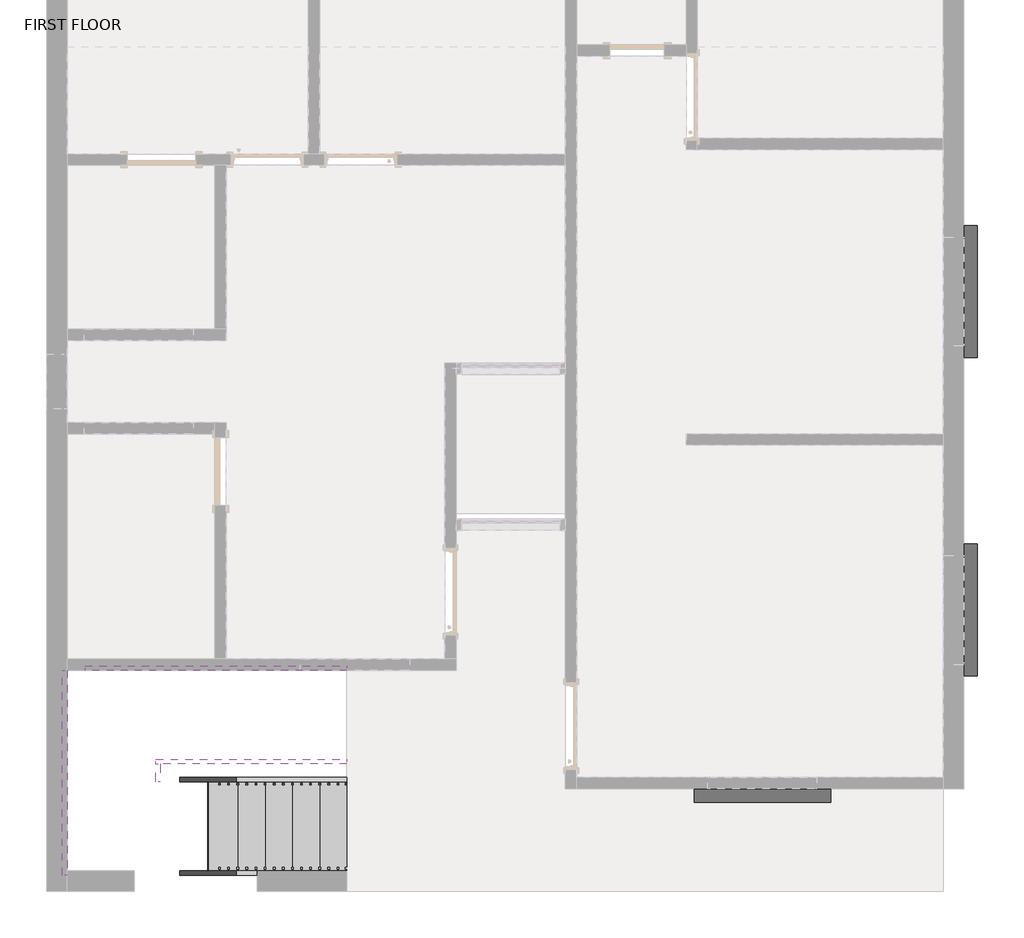
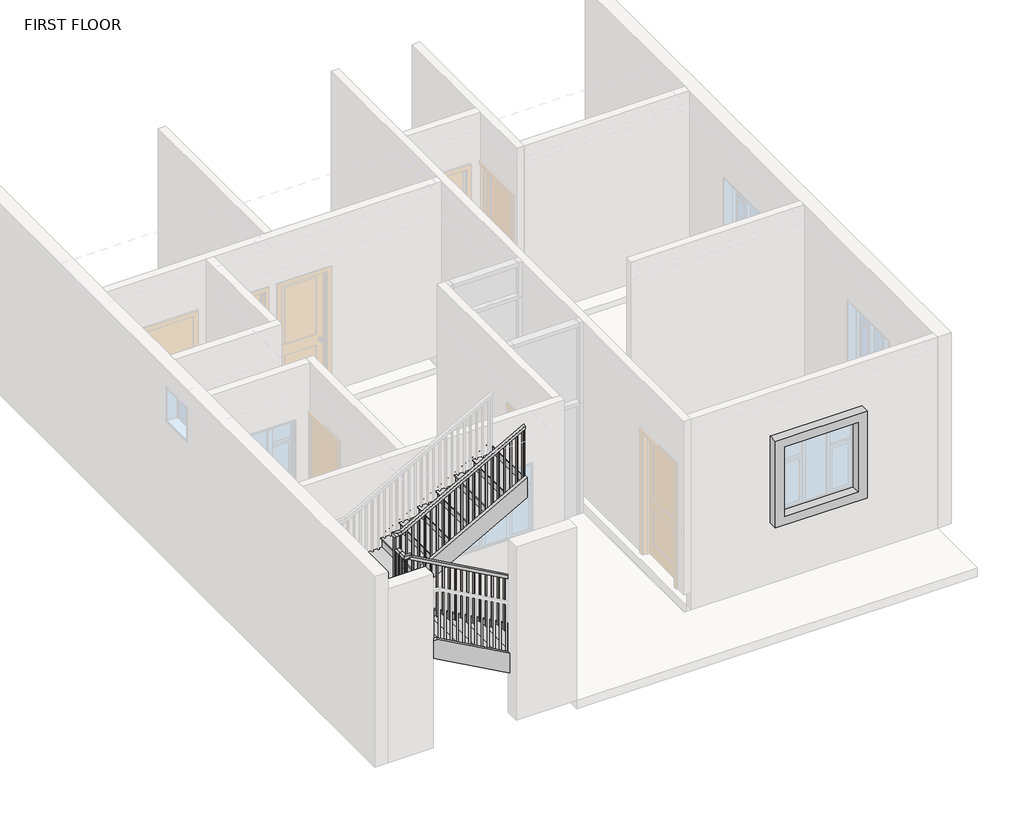
# One storey, part 3 of 3: 6 members, 3 proxies, 1 railing, 1 stair flight.
"""IFC4 building model written with IfcOpenShell, lengths in millimetres."""

from ifc_helpers import new_model, si_unit, frame, origin, place, context, project, spatial, polyline, outline, extrude, faceted_brep, transform, mapped, element, save
from components import generic_models_3_generic_models_3_0ad4c425, generic_models_6_generic_models_6_ceaf88ca, stair_flight_128b20ea

model = new_model("IFC4")

# Units and contexts
model_context = context("Model", 3, world=origin())
ifc_project = project(units=[si_unit("LENGTHUNIT", "METRE", prefix="MILLI")], contexts=[model_context])

# Site, building, storey
site = spatial("IfcSite", under=ifc_project)
building = spatial("IfcBuilding", under=site)
storey = spatial("IfcBuildingStorey", under=building, Name="FIRST FLOOR", Elevation=3352.8)

# Proxies
placement = place(None, origin())
generic_models_3_generic_models_3_shape = generic_models_3_generic_models_3_0ad4c425(model_context)
element("IfcBuildingElementProxy", 1, Name="Generic Models 3 : Generic Models 3", ObjectType="Generic Models 3 : Generic Models 3", at=placement, inside=storey, context=model_context, shape_type="MappedRepresentation", body=[
    mapped(generic_models_3_generic_models_3_shape, transform((0.0, 0.0, 0.0), x_axis=(1.0, 0.0, 0.0), y_axis=(0.0, 1.0, 0.0), z_axis=(0.0, 0.0, 1.0))),
])
generic_models_6_generic_models_6_shape = generic_models_6_generic_models_6_ceaf88ca(model_context)
element("IfcBuildingElementProxy", 2, Name="Generic Models 6 : Generic Models 6", ObjectType="Generic Models 6 : Generic Models 6", at=placement, inside=storey, context=model_context, shape_type="MappedRepresentation", body=[
    mapped(generic_models_6_generic_models_6_shape, transform((0.0, 0.0, 0.0), x_axis=(1.0, 0.0, 0.0), y_axis=(0.0, 1.0, 0.0), z_axis=(0.0, 0.0, 1.0))),
])
element("IfcBuildingElementProxy", 3, Name="Generic Models 7 : Generic Models 6", ObjectType="Generic Models 7 : Generic Models 6", at=placement, inside=storey, context=model_context, shape_type="MappedRepresentation", body=[
    mapped(generic_models_6_generic_models_6_shape, transform((0.0, 3556.0, 0.0), x_axis=(1.0, 0.0, 0.0), y_axis=(0.0, 1.0, 0.0), z_axis=(0.0, 0.0, 1.0))),
])

# Members
element("IfcMember", 4, ObjectType="Stringer - 2\" Width", at=placement, inside=storey, context=model_context, shape_type="SweptSolid", body=[
    extrude(outline(polyline([(3657.6, -11636.5023867), (3865.1983948, -11636.5023867), (5088.4666667, -13838.3852761), (5088.4666667, -14466.0068895), (3657.6, -11890.4468895), (3657.6, -11636.5023867)])), frame((0.0, -2807.5499863, 0.0), z_axis=(0.0, 1.0, 0.0), x_axis=(0.0, 0.0, 1.0)), (0.0, 0.0, 1.0), 50.8),
])
element("IfcMember", 5, ObjectType="Stringer - 2\" Width", at=placement, inside=storey, context=model_context, shape_type="SweptSolid", body=[
    extrude(outline(polyline([(-14760.7023867, -2807.5499863), (-14811.5023867, -2807.5499863), (-14811.5023867, -521.5499863), (-14760.7023867, -521.5499863), (-14760.7023867, -2807.5499863)])), frame((0.0, 0.0, 4783.6666667), z_axis=(0.0, 0.0, 1.0), x_axis=(1.0, 0.0, 0.0)), (0.0, 0.0, 1.0), 304.8),
])
element("IfcMember", 6, ObjectType="Stringer - 2\" Width", at=placement, inside=storey, context=model_context, shape_type="SweptSolid", body=[
    extrude(outline(polyline([(4783.6666667, -13927.6378839), (6056.5197207, -11636.5023867), (6405.1983948, -11636.5023867), (4783.6666667, -14555.2594973), (4783.6666667, -13927.6378839)])), frame((0.0, -521.5499863, 0.0), z_axis=(0.0, 1.0, 0.0), x_axis=(0.0, 0.0, 1.0)), (0.0, 0.0, 1.0), 50.8),
])
element("IfcMember", 7, ObjectType="Stringer - 2\" Width", at=placement, inside=storey, context=model_context, shape_type="SweptSolid", body=[
    extrude(outline(polyline([(3657.6, -11636.5023867), (3865.1983948, -11636.5023867), (5022.3095059, -13719.3023867), (4673.6308318, -13719.3023867), (3657.6, -11890.4468895), (3657.6, -11636.5023867)])), frame((0.0, -1766.1499863, 0.0), z_axis=(0.0, 1.0, 0.0), x_axis=(0.0, 0.0, 1.0)), (0.0, 0.0, 1.0), 50.8),
])
element("IfcMember", 8, ObjectType="Stringer - 2\" Width", at=placement, inside=storey, context=model_context, shape_type="SweptSolid", body=[
    extrude(outline(polyline([(-13719.3023867, -1766.1499863), (-13770.1023867, -1766.1499863), (-13770.1023867, -1562.9499863), (-13719.3023867, -1562.9499863), (-13719.3023867, -1766.1499863)])), frame((0.0, 0.0, 4783.6666667), z_axis=(0.0, 0.0, 1.0), x_axis=(1.0, 0.0, 0.0)), (0.0, 0.0, 1.0), 304.8),
])
element("IfcMember", 9, ObjectType="Stringer - 2\" Width", at=placement, inside=storey, context=model_context, shape_type="SweptSolid", body=[
    extrude(outline(polyline([(5219.8650614, -13770.1023867), (4871.1863873, -13770.1023867), (6056.5197207, -11636.5023867), (6405.1983948, -11636.5023867), (5219.8650614, -13770.1023867)])), frame((0.0, -1562.9499863, 0.0), z_axis=(0.0, 1.0, 0.0), x_axis=(0.0, 0.0, 1.0)), (0.0, 0.0, 1.0), 50.8),
])

# Railing
element("IfcRailing", 10, ObjectType="Handrail - Rectangular", at=placement, inside=storey, context=model_context, shape_type="SolidModel", body=[
    faceted_brep([(-11636.5023867, -1816.9499863, 4741.3333333), (-11636.5023867, -1816.9499863, 4683.220221), (-11636.5023867, -1766.1499863, 4683.220221), (-11636.5023867, -1766.1499863, 4741.3333333), (-13693.9023867, -1816.9499863, 5884.3333333), (-13744.7023867, -1816.9499863, 5854.4424432), (-13744.7023867, -1766.1499863, 5854.4424432), (-13693.9023867, -1766.1499863, 5884.3333333), (-13693.9023867, -1816.9499863, 5926.6666667), (-13744.7023867, -1816.9499863, 5875.8666667), (-13744.7023867, -1766.1499863, 5875.8666667), (-13693.9023867, -1766.1499863, 5926.6666667), (-13820.9023867, -1816.9499863, 5926.6666667), (-13820.9023867, -1816.9499863, 5875.8666667), (-13770.1023867, -1766.1499863, 5875.8666667), (-13770.1023867, -1766.1499863, 5926.6666667), (-13820.9023867, -1689.9499863, 5926.6666667), (-13820.9023867, -1689.9499863, 5875.8666667), (-13770.1023867, -1689.9499863, 5875.8666667), (-13770.1023867, -1689.9499863, 5926.6666667), (-13820.9023867, -1588.3499863, 5926.6666667), (-13820.9023867, -1537.5499863, 5875.8666667), (-13770.1023867, -1537.5499863, 5875.8666667), (-13770.1023867, -1588.3499863, 5926.6666667), (-13820.9023867, -1588.3499863, 6138.3333333), (-13820.9023867, -1537.5499863, 6087.5333333), (-13770.1023867, -1537.5499863, 6087.5333333), (-13770.1023867, -1588.3499863, 6138.3333333), (-13820.9023867, -1461.3499863, 6138.3333333), (-13820.9023867, -1461.3499863, 6087.5333333), (-13770.1023867, -1512.1499863, 6087.5333333), (-13770.1023867, -1512.1499863, 6138.3333333), (-13693.9023867, -1461.3499863, 6138.3333333), (-13680.7387844, -1461.3499863, 6087.5333333), (-13680.7387844, -1512.1499863, 6087.5333333), (-13693.9023867, -1512.1499863, 6138.3333333), (-11636.5023867, -1461.3499863, 7281.3333333), (-11636.5023867, -1512.1499863, 7281.3333333), (-11636.5023867, -1512.1499863, 7223.220221), (-11636.5023867, -1461.3499863, 7223.220221)], [[[0, 1, 2, 3]], [[1, 0, 4, 5]], [[2, 1, 5, 6]], [[3, 2, 6, 7]], [[0, 3, 7, 4]], [[5, 4, 8, 9]], [[6, 5, 9, 10]], [[7, 6, 10, 11]], [[4, 7, 11, 8]], [[9, 8, 12, 13]], [[10, 9, 13, 14]], [[11, 10, 14, 15]], [[8, 11, 15, 12]], [[13, 12, 16, 17]], [[14, 13, 17, 18]], [[15, 14, 18, 19]], [[12, 15, 19, 16]], [[17, 16, 20, 21]], [[18, 17, 21, 22]], [[19, 18, 22, 23]], [[16, 19, 23, 20]], [[21, 20, 24, 25]], [[22, 21, 25, 26]], [[23, 22, 26, 27]], [[20, 23, 27, 24]], [[25, 24, 28, 29]], [[26, 25, 29, 30]], [[27, 26, 30, 31]], [[24, 27, 31, 28]], [[29, 28, 32, 33]], [[30, 29, 33, 34]], [[31, 30, 34, 35]], [[28, 31, 35, 32]], [[36, 37, 38, 39]], [[33, 32, 36, 39]], [[34, 33, 39, 38]], [[35, 34, 38, 37]], [[32, 35, 37, 36]]]),
    extrude(outline(polyline([(7214.4007765, -11652.3773867), (7203.8174432, -11671.4273867), (6197.6, -11671.4273867), (6197.6, -11652.3773867), (7214.4007765, -11652.3773867)])), frame((0.0, -1496.2749863, 0.0), z_axis=(0.0, 1.0, 0.0), x_axis=(0.0, 0.0, 1.0)), (0.0, 0.0, 1.0), 19.05),
    extrude(outline(polyline([(7157.9563321, -11753.9773867), (7147.3729988, -11773.0273867), (6197.6, -11773.0273867), (6197.6, -11753.9773867), (7157.9563321, -11753.9773867)])), frame((0.0, -1496.2749863, 0.0), z_axis=(0.0, 1.0, 0.0), x_axis=(0.0, 0.0, 1.0)), (0.0, 0.0, 1.0), 19.05),
    extrude(outline(polyline([(7101.5118876, -11855.5773867), (7090.9285543, -11874.6273867), (6197.6, -11874.6273867), (6197.6, -11855.5773867), (7101.5118876, -11855.5773867)])), frame((0.0, -1496.2749863, 0.0), z_axis=(0.0, 1.0, 0.0), x_axis=(0.0, 0.0, 1.0)), (0.0, 0.0, 1.0), 19.05),
    extrude(outline(polyline([(7045.0674432, -11957.1773867), (7034.4841099, -11976.2273867), (6028.2666667, -11976.2273867), (6028.2666667, -11957.1773867), (7045.0674432, -11957.1773867)])), frame((0.0, -1496.2749863, 0.0), z_axis=(0.0, 1.0, 0.0), x_axis=(0.0, 0.0, 1.0)), (0.0, 0.0, 1.0), 19.05),
    extrude(outline(polyline([(6988.6229988, -12058.7773867), (6978.0396654, -12077.8273867), (6028.2666667, -12077.8273867), (6028.2666667, -12058.7773867), (6988.6229988, -12058.7773867)])), frame((0.0, -1496.2749863, 0.0), z_axis=(0.0, 1.0, 0.0), x_axis=(0.0, 0.0, 1.0)), (0.0, 0.0, 1.0), 19.05),
    extrude(outline(polyline([(6932.1785543, -12160.3773867), (6921.595221, -12179.4273867), (6028.2666667, -12179.4273867), (6028.2666667, -12160.3773867), (6932.1785543, -12160.3773867)])), frame((0.0, -1496.2749863, 0.0), z_axis=(0.0, 1.0, 0.0), x_axis=(0.0, 0.0, 1.0)), (0.0, 0.0, 1.0), 19.05),
    extrude(outline(polyline([(6875.7341099, -12261.9773867), (6865.1507765, -12281.0273867), (5858.9333333, -12281.0273867), (5858.9333333, -12261.9773867), (6875.7341099, -12261.9773867)])), frame((0.0, -1496.2749863, 0.0), z_axis=(0.0, 1.0, 0.0), x_axis=(0.0, 0.0, 1.0)), (0.0, 0.0, 1.0), 19.05),
    extrude(outline(polyline([(6819.2896654, -12363.5773867), (6808.7063321, -12382.6273867), (5858.9333333, -12382.6273867), (5858.9333333, -12363.5773867), (6819.2896654, -12363.5773867)])), frame((0.0, -1496.2749863, 0.0), z_axis=(0.0, 1.0, 0.0), x_axis=(0.0, 0.0, 1.0)), (0.0, 0.0, 1.0), 19.05),
    extrude(outline(polyline([(6762.845221, -12465.1773867), (6752.2618876, -12484.2273867), (5858.9333333, -12484.2273867), (5858.9333333, -12465.1773867), (6762.845221, -12465.1773867)])), frame((0.0, -1496.2749863, 0.0), z_axis=(0.0, 1.0, 0.0), x_axis=(0.0, 0.0, 1.0)), (0.0, 0.0, 1.0), 19.05),
    extrude(outline(polyline([(6706.4007765, -12566.7773867), (6695.8174432, -12585.8273867), (5689.6, -12585.8273867), (5689.6, -12566.7773867), (6706.4007765, -12566.7773867)])), frame((0.0, -1496.2749863, 0.0), z_axis=(0.0, 1.0, 0.0), x_axis=(0.0, 0.0, 1.0)), (0.0, 0.0, 1.0), 19.05),
    extrude(outline(polyline([(6649.9563321, -12668.3773867), (6639.3729988, -12687.4273867), (5689.6, -12687.4273867), (5689.6, -12668.3773867), (6649.9563321, -12668.3773867)])), frame((0.0, -1496.2749863, 0.0), z_axis=(0.0, 1.0, 0.0), x_axis=(0.0, 0.0, 1.0)), (0.0, 0.0, 1.0), 19.05),
    extrude(outline(polyline([(6593.5118876, -12769.9773867), (6582.9285543, -12789.0273867), (5689.6, -12789.0273867), (5689.6, -12769.9773867), (6593.5118876, -12769.9773867)])), frame((0.0, -1496.2749863, 0.0), z_axis=(0.0, 1.0, 0.0), x_axis=(0.0, 0.0, 1.0)), (0.0, 0.0, 1.0), 19.05),
    extrude(outline(polyline([(6537.0674432, -12871.5773867), (6526.4841099, -12890.6273867), (5520.2666667, -12890.6273867), (5520.2666667, -12871.5773867), (6537.0674432, -12871.5773867)])), frame((0.0, -1496.2749863, 0.0), z_axis=(0.0, 1.0, 0.0), x_axis=(0.0, 0.0, 1.0)), (0.0, 0.0, 1.0), 19.05),
    extrude(outline(polyline([(6480.6229988, -12973.1773867), (6470.0396654, -12992.2273867), (5520.2666667, -12992.2273867), (5520.2666667, -12973.1773867), (6480.6229988, -12973.1773867)])), frame((0.0, -1496.2749863, 0.0), z_axis=(0.0, 1.0, 0.0), x_axis=(0.0, 0.0, 1.0)), (0.0, 0.0, 1.0), 19.05),
    extrude(outline(polyline([(6424.1785543, -13074.7773867), (6413.595221, -13093.8273867), (5520.2666667, -13093.8273867), (5520.2666667, -13074.7773867), (6424.1785543, -13074.7773867)])), frame((0.0, -1496.2749863, 0.0), z_axis=(0.0, 1.0, 0.0), x_axis=(0.0, 0.0, 1.0)), (0.0, 0.0, 1.0), 19.05),
    extrude(outline(polyline([(6367.7341099, -13176.3773867), (6357.1507765, -13195.4273867), (5350.9333333, -13195.4273867), (5350.9333333, -13176.3773867), (6367.7341099, -13176.3773867)])), frame((0.0, -1496.2749863, 0.0), z_axis=(0.0, 1.0, 0.0), x_axis=(0.0, 0.0, 1.0)), (0.0, 0.0, 1.0), 19.05),
    extrude(outline(polyline([(6311.2896654, -13277.9773867), (6300.7063321, -13297.0273867), (5350.9333333, -13297.0273867), (5350.9333333, -13277.9773867), (6311.2896654, -13277.9773867)])), frame((0.0, -1496.2749863, 0.0), z_axis=(0.0, 1.0, 0.0), x_axis=(0.0, 0.0, 1.0)), (0.0, 0.0, 1.0), 19.05),
    extrude(outline(polyline([(6254.845221, -13379.5773867), (6244.2618876, -13398.6273867), (5350.9333333, -13398.6273867), (5350.9333333, -13379.5773867), (6254.845221, -13379.5773867)])), frame((0.0, -1496.2749863, 0.0), z_axis=(0.0, 1.0, 0.0), x_axis=(0.0, 0.0, 1.0)), (0.0, 0.0, 1.0), 19.05),
    extrude(outline(polyline([(6198.4007765, -13481.1773867), (6187.8174432, -13500.2273867), (5181.6, -13500.2273867), (5181.6, -13481.1773867), (6198.4007765, -13481.1773867)])), frame((0.0, -1496.2749863, 0.0), z_axis=(0.0, 1.0, 0.0), x_axis=(0.0, 0.0, 1.0)), (0.0, 0.0, 1.0), 19.05),
    extrude(outline(polyline([(6141.9563321, -13582.7773867), (6131.3729988, -13601.8273867), (5181.6, -13601.8273867), (5181.6, -13582.7773867), (6141.9563321, -13582.7773867)])), frame((0.0, -1496.2749863, 0.0), z_axis=(0.0, 1.0, 0.0), x_axis=(0.0, 0.0, 1.0)), (0.0, 0.0, 1.0), 19.05),
    extrude(outline(polyline([(6085.5118876, -13684.3773867), (6074.9285543, -13703.4273867), (5181.6, -13703.4273867), (5181.6, -13684.3773867), (6085.5118876, -13684.3773867)])), frame((0.0, -1496.2749863, 0.0), z_axis=(0.0, 1.0, 0.0), x_axis=(0.0, 0.0, 1.0)), (0.0, 0.0, 1.0), 19.05),
    extrude(outline(polyline([(-13785.9773867, -1597.8749863), (-13805.0273867, -1597.8749863), (-13805.0273867, -1578.8249863), (-13785.9773867, -1578.8249863), (-13785.9773867, -1597.8749863)])), frame((0.0, 0.0, 5012.2666667), z_axis=(0.0, 0.0, 1.0), x_axis=(1.0, 0.0, 0.0)), (0.0, 0.0, 1.0), 863.6),
    extrude(outline(polyline([(-13785.9773867, -1699.4749863), (-13805.0273867, -1699.4749863), (-13805.0273867, -1680.4249863), (-13785.9773867, -1680.4249863), (-13785.9773867, -1699.4749863)])), frame((0.0, 0.0, 5012.2666667), z_axis=(0.0, 0.0, 1.0), x_axis=(1.0, 0.0, 0.0)), (0.0, 0.0, 1.0), 863.6),
    extrude(outline(polyline([(-13760.5773867, -1782.0249863), (-13760.5773867, -1801.0749863), (-13779.6273867, -1801.0749863), (-13779.6273867, -1782.0249863), (-13760.5773867, -1782.0249863)])), frame((0.0, 0.0, 5012.2666667), z_axis=(0.0, 0.0, 1.0), x_axis=(1.0, 0.0, 0.0)), (0.0, 0.0, 1.0), 863.6),
    extrude(outline(polyline([(5806.8174432, -13658.9773867), (5817.4007765, -13678.0273867), (4842.9333333, -13678.0273867), (4842.9333333, -13658.9773867), (5806.8174432, -13658.9773867)])), frame((0.0, -1801.0749863, 0.0), z_axis=(0.0, 1.0, 0.0), x_axis=(0.0, 0.0, 1.0)), (0.0, 0.0, 1.0), 19.05),
    extrude(outline(polyline([(5750.3729988, -13557.3773867), (5760.9563321, -13576.4273867), (4842.9333333, -13576.4273867), (4842.9333333, -13557.3773867), (5750.3729988, -13557.3773867)])), frame((0.0, -1801.0749863, 0.0), z_axis=(0.0, 1.0, 0.0), x_axis=(0.0, 0.0, 1.0)), (0.0, 0.0, 1.0), 19.05),
    extrude(outline(polyline([(5693.9285543, -13455.7773867), (5704.5118876, -13474.8273867), (4842.9333333, -13474.8273867), (4842.9333333, -13455.7773867), (5693.9285543, -13455.7773867)])), frame((0.0, -1801.0749863, 0.0), z_axis=(0.0, 1.0, 0.0), x_axis=(0.0, 0.0, 1.0)), (0.0, 0.0, 1.0), 19.05),
    extrude(outline(polyline([(5637.4841099, -13354.1773867), (5648.0674432, -13373.2273867), (4673.6, -13373.2273867), (4673.6, -13354.1773867), (5637.4841099, -13354.1773867)])), frame((0.0, -1801.0749863, 0.0), z_axis=(0.0, 1.0, 0.0), x_axis=(0.0, 0.0, 1.0)), (0.0, 0.0, 1.0), 19.05),
    extrude(outline(polyline([(5581.0396654, -13252.5773867), (5591.6229988, -13271.6273867), (4673.6, -13271.6273867), (4673.6, -13252.5773867), (5581.0396654, -13252.5773867)])), frame((0.0, -1801.0749863, 0.0), z_axis=(0.0, 1.0, 0.0), x_axis=(0.0, 0.0, 1.0)), (0.0, 0.0, 1.0), 19.05),
    extrude(outline(polyline([(5524.595221, -13150.9773867), (5535.1785543, -13170.0273867), (4673.6, -13170.0273867), (4673.6, -13150.9773867), (5524.595221, -13150.9773867)])), frame((0.0, -1801.0749863, 0.0), z_axis=(0.0, 1.0, 0.0), x_axis=(0.0, 0.0, 1.0)), (0.0, 0.0, 1.0), 19.05),
    extrude(outline(polyline([(5468.1507765, -13049.3773867), (5478.7341099, -13068.4273867), (4504.2666667, -13068.4273867), (4504.2666667, -13049.3773867), (5468.1507765, -13049.3773867)])), frame((0.0, -1801.0749863, 0.0), z_axis=(0.0, 1.0, 0.0), x_axis=(0.0, 0.0, 1.0)), (0.0, 0.0, 1.0), 19.05),
    extrude(outline(polyline([(5411.7063321, -12947.7773867), (5422.2896654, -12966.8273867), (4504.2666667, -12966.8273867), (4504.2666667, -12947.7773867), (5411.7063321, -12947.7773867)])), frame((0.0, -1801.0749863, 0.0), z_axis=(0.0, 1.0, 0.0), x_axis=(0.0, 0.0, 1.0)), (0.0, 0.0, 1.0), 19.05),
    extrude(outline(polyline([(5355.2618876, -12846.1773867), (5365.845221, -12865.2273867), (4504.2666667, -12865.2273867), (4504.2666667, -12846.1773867), (5355.2618876, -12846.1773867)])), frame((0.0, -1801.0749863, 0.0), z_axis=(0.0, 1.0, 0.0), x_axis=(0.0, 0.0, 1.0)), (0.0, 0.0, 1.0), 19.05),
    extrude(outline(polyline([(5298.8174432, -12744.5773867), (5309.4007765, -12763.6273867), (4334.9333333, -12763.6273867), (4334.9333333, -12744.5773867), (5298.8174432, -12744.5773867)])), frame((0.0, -1801.0749863, 0.0), z_axis=(0.0, 1.0, 0.0), x_axis=(0.0, 0.0, 1.0)), (0.0, 0.0, 1.0), 19.05),
    extrude(outline(polyline([(5242.3729988, -12642.9773867), (5252.9563321, -12662.0273867), (4334.9333333, -12662.0273867), (4334.9333333, -12642.9773867), (5242.3729988, -12642.9773867)])), frame((0.0, -1801.0749863, 0.0), z_axis=(0.0, 1.0, 0.0), x_axis=(0.0, 0.0, 1.0)), (0.0, 0.0, 1.0), 19.05),
    extrude(outline(polyline([(5185.9285543, -12541.3773867), (5196.5118876, -12560.4273867), (4334.9333333, -12560.4273867), (4334.9333333, -12541.3773867), (5185.9285543, -12541.3773867)])), frame((0.0, -1801.0749863, 0.0), z_axis=(0.0, 1.0, 0.0), x_axis=(0.0, 0.0, 1.0)), (0.0, 0.0, 1.0), 19.05),
    extrude(outline(polyline([(5129.4841099, -12439.7773867), (5140.0674432, -12458.8273867), (4165.6, -12458.8273867), (4165.6, -12439.7773867), (5129.4841099, -12439.7773867)])), frame((0.0, -1801.0749863, 0.0), z_axis=(0.0, 1.0, 0.0), x_axis=(0.0, 0.0, 1.0)), (0.0, 0.0, 1.0), 19.05),
    extrude(outline(polyline([(5073.0396654, -12338.1773867), (5083.6229988, -12357.2273867), (4165.6, -12357.2273867), (4165.6, -12338.1773867), (5073.0396654, -12338.1773867)])), frame((0.0, -1801.0749863, 0.0), z_axis=(0.0, 1.0, 0.0), x_axis=(0.0, 0.0, 1.0)), (0.0, 0.0, 1.0), 19.05),
    extrude(outline(polyline([(5016.595221, -12236.5773867), (5027.1785543, -12255.6273867), (4165.6, -12255.6273867), (4165.6, -12236.5773867), (5016.595221, -12236.5773867)])), frame((0.0, -1801.0749863, 0.0), z_axis=(0.0, 1.0, 0.0), x_axis=(0.0, 0.0, 1.0)), (0.0, 0.0, 1.0), 19.05),
    extrude(outline(polyline([(4960.1507765, -12134.9773867), (4970.7341099, -12154.0273867), (3996.2666667, -12154.0273867), (3996.2666667, -12134.9773867), (4960.1507765, -12134.9773867)])), frame((0.0, -1801.0749863, 0.0), z_axis=(0.0, 1.0, 0.0), x_axis=(0.0, 0.0, 1.0)), (0.0, 0.0, 1.0), 19.05),
    extrude(outline(polyline([(4903.7063321, -12033.3773867), (4914.2896654, -12052.4273867), (3996.2666667, -12052.4273867), (3996.2666667, -12033.3773867), (4903.7063321, -12033.3773867)])), frame((0.0, -1801.0749863, 0.0), z_axis=(0.0, 1.0, 0.0), x_axis=(0.0, 0.0, 1.0)), (0.0, 0.0, 1.0), 19.05),
    extrude(outline(polyline([(4847.2618876, -11931.7773867), (4857.845221, -11950.8273867), (3996.2666667, -11950.8273867), (3996.2666667, -11931.7773867), (4847.2618876, -11931.7773867)])), frame((0.0, -1801.0749863, 0.0), z_axis=(0.0, 1.0, 0.0), x_axis=(0.0, 0.0, 1.0)), (0.0, 0.0, 1.0), 19.05),
    extrude(outline(polyline([(4790.8174432, -11830.1773867), (4801.4007765, -11849.2273867), (3826.9333333, -11849.2273867), (3826.9333333, -11830.1773867), (4790.8174432, -11830.1773867)])), frame((0.0, -1801.0749863, 0.0), z_axis=(0.0, 1.0, 0.0), x_axis=(0.0, 0.0, 1.0)), (0.0, 0.0, 1.0), 19.05),
    extrude(outline(polyline([(4734.3729988, -11728.5773867), (4744.9563321, -11747.6273867), (3826.9333333, -11747.6273867), (3826.9333333, -11728.5773867), (4734.3729988, -11728.5773867)])), frame((0.0, -1801.0749863, 0.0), z_axis=(0.0, 1.0, 0.0), x_axis=(0.0, 0.0, 1.0)), (0.0, 0.0, 1.0), 19.05),
    extrude(outline(polyline([(-13785.9773867, -1496.2749863), (-13805.0273867, -1496.2749863), (-13805.0273867, -1477.2249863), (-13785.9773867, -1477.2249863), (-13785.9773867, -1496.2749863)])), frame((0.0, 0.0, 5012.2666667), z_axis=(0.0, 0.0, 1.0), x_axis=(1.0, 0.0, 0.0)), (0.0, 0.0, 1.0), 1075.2666667),
    extrude(outline(polyline([(-13785.9773867, -1782.0249863), (-13785.9773867, -1801.0749863), (-13805.0273867, -1801.0749863), (-13805.0273867, -1782.0249863), (-13785.9773867, -1782.0249863)])), frame((0.0, 0.0, 5012.2666667), z_axis=(0.0, 0.0, 1.0), x_axis=(1.0, 0.0, 0.0)), (0.0, 0.0, 1.0), 863.6),
    extrude(outline(polyline([(7223.220221, -11636.5023867), (7212.6368876, -11655.5523867), (6197.6, -11655.5523867), (6197.6, -11636.5023867), (7223.220221, -11636.5023867)])), frame((0.0, -1496.2749863, 0.0), z_axis=(0.0, 1.0, 0.0), x_axis=(0.0, 0.0, 1.0)), (0.0, 0.0, 1.0), 19.05),
    extrude(outline(polyline([(4683.220221, -11636.5023867), (4693.8035543, -11655.5523867), (3826.9333333, -11655.5523867), (3826.9333333, -11636.5023867), (4683.220221, -11636.5023867)])), frame((0.0, -1801.0749863, 0.0), z_axis=(0.0, 1.0, 0.0), x_axis=(0.0, 0.0, 1.0)), (0.0, 0.0, 1.0), 19.05),
])

# Stair flight
stair_flight_shape = stair_flight_128b20ea(model_context)
element("IfcStairFlight", 11, ObjectType="2\" Tread 1\" Nosing 1/4\" Riser", at=placement, inside=storey, context=model_context, shape_type="MappedRepresentation", body=[
    mapped(stair_flight_shape, transform((0.0, 0.0, 0.0), x_axis=(1.0, 0.0, 0.0), y_axis=(0.0, 1.0, 0.0), z_axis=(0.0, 0.0, 1.0))),
])

save(model, "model.ifc")

# Revit data of these elements
# Type "Handrail - Rectangular"
#   Assembly Code = "C2010400"
#   built-in parameter 1008612 = 0.0416667 (stored number, unit not read)
#   built-in parameter 1008611 = 0.0416667 (stored number, unit not read)
#   built-in parameter 1008609 = 0.333333 (stored number, unit not read)
#   built-in parameter 1008604 = 0.166667 (stored number, unit not read)
#   built-in parameter 1008603 = 0.166667 (stored number, unit not read)
#   Railing Height = 3' - 0"
#   built-in parameter 1008630 = 2
#   built-in parameter 1008610 = 2
#   built-in parameter 1008618 = Baluster - Square : 3/4"
# Element 1 (IfcBuildingElementProxy, "Generic Models 3 : Generic Models 3")
#   Phase Created = New Construction
#   Materials on its faces: "accent wall"
# Element 2 (IfcBuildingElementProxy, "Generic Models 6 : Generic Models 6")
#   Phase Created = New Construction
#   Materials on its faces: "accent wall"
# Element 3 (IfcBuildingElementProxy, "Generic Models 7 : Generic Models 6")
#   Phase Created = New Construction
#   Materials on its faces: "accent wall"
# Elements 4, 5, 6, 7, 8, 9 (IfcMember, "Stringer - 2\" Width")
#   Phase Created = New Construction
# Element 10 (IfcRailing, "Handrail - Rectangular")
#   Phase Created = New Construction
# Element 11 (IfcStairFlight, "2\" Tread 1\" Nosing 1/4\" Riser")
#   Phase Created = New Construction
# Materials
#   "accent wall": class "Generic", colour RGB 120 120 120, transparency 0, Cost = 0
